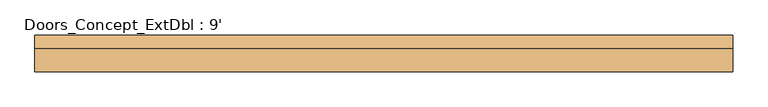
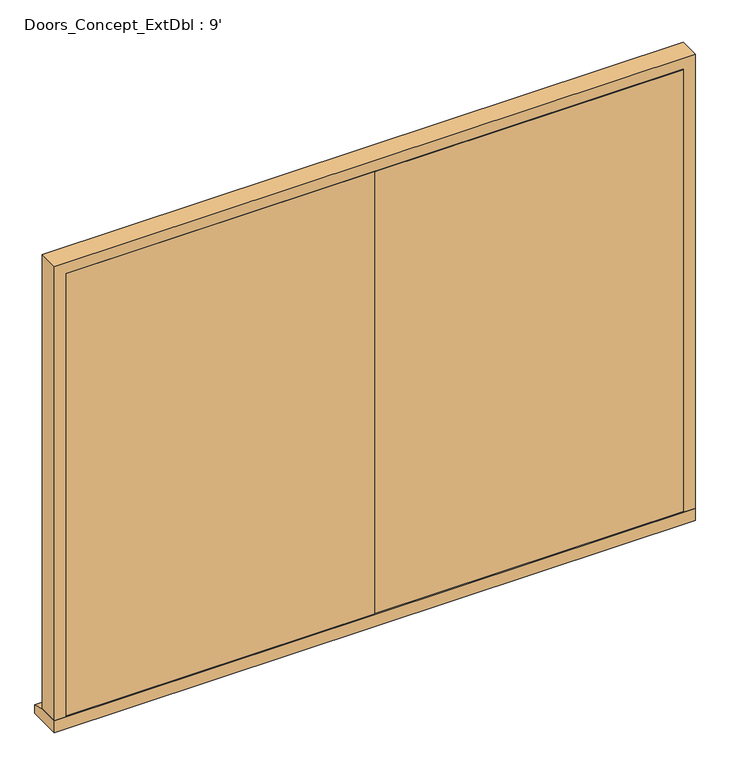
"""IFC4 building model written with IfcOpenShell, lengths in millimetres: door geometry, Doors_Concept_ExtDbl : 9'."""

from ifc_helpers import new_model, si_unit, frame, origin, place, context, project, spatial, polyline, outline, extrude, faceted_brep, source, transform, mapped, element, save


def doors_concept_extdbl_9_6115d45a(model_context):
    return source(origin(), model_context, "Body", "SolidModel", [
        faceted_brep([(1301.1, 74.06, 54.5), (1371.6, 74.06, 54.5), (1371.6, -14.94, 54.5), (1323.1, -14.94, 54.5), (1323.1, 32.06, 54.5), (1301.1, 32.06, 54.5), (1301.1, 74.06, 2039.5), (-1301.1, 74.06, 2039.5), (-1301.1, 74.06, 54.5), (-1371.6, 74.06, 54.5), (-1371.6, 74.06, 2110.0), (1371.6, 74.06, 2110.0), (1371.6, -14.94, 2110.0), (-1371.6, -14.94, 2110.0), (-1371.6, -14.94, 54.5), (-1323.1, -14.94, 54.5), (-1323.1, -14.94, 2061.5), (1323.1, -14.94, 2061.5), (1323.1, 32.06, 2061.5), (-1323.1, 32.06, 2061.5), (-1323.1, 32.06, 54.5), (-1301.1, 32.06, 54.5), (-1301.1, 32.06, 2039.5), (1301.1, 32.06, 2039.5)], [[[0, 1, 2, 3, 4, 5]], [[1, 0, 6, 7, 8, 9, 10, 11]], [[2, 1, 11, 12]], [[3, 2, 12, 13, 14, 15, 16, 17]], [[4, 3, 17, 18]], [[5, 4, 18, 19, 20, 21, 22, 23]], [[0, 5, 23, 6]], [[7, 22, 21, 8]], [[8, 21, 20, 15, 14, 9]], [[13, 10, 9, 14]], [[19, 16, 15, 20]], [[12, 11, 10, 13]], [[18, 17, 16, 19]], [[6, 23, 22, 7]]]),
        extrude(outline(polyline([(1320.1, -14.94), (1.5, -14.94), (1.5, 29.06), (1320.1, 29.06), (1320.1, -14.94)])), frame((0.0, 0.0, 58.5), z_axis=(0.0, 0.0, 1.0), x_axis=(1.0, 0.0, 0.0)), (0.0, 0.0, 1.0), 2000.0),
        extrude(outline(polyline([(-1.5, -14.94), (-1320.1, -14.94), (-1320.1, 29.06), (-1.5, 29.06), (-1.5, -14.94)])), frame((0.0, 0.0, 58.5), z_axis=(0.0, 0.0, 1.0), x_axis=(1.0, 0.0, 0.0)), (0.0, 0.0, 1.0), 2000.0),
        extrude(outline(polyline([(-14.94, 0.0), (-14.94, 54.5), (74.06, 54.5), (129.06, 38.5947221), (129.06, 0.0), (-14.94, 0.0)])), frame((-1371.6, 0.0, 0.0), z_axis=(1.0, 0.0, 0.0), x_axis=(0.0, 1.0, 0.0)), (0.0, 0.0, 1.0), 2743.2),
    ])


if __name__ == "__main__":
    model = new_model("IFC4")
    model_context = context("Model", 3, world=origin())
    ifc_project = project(units=[si_unit("LENGTHUNIT", "METRE", prefix="MILLI")], contexts=[model_context])
    site = spatial("IfcSite", under=ifc_project)
    building = spatial("IfcBuilding", under=site)
    placement = place(None, origin())
    doors_concept_extdbl_9_shape = doors_concept_extdbl_9_6115d45a(model_context)
    element("IfcDoor", 1, ObjectType="Doors_Concept_ExtDbl : 9'", at=placement, inside=building, context=model_context, shape_type="MappedRepresentation", body=[
        mapped(doors_concept_extdbl_9_shape, transform((0.0, 0.0, 0.0), x_axis=(1.0, 0.0, 0.0), y_axis=(0.0, 1.0, 0.0), z_axis=(0.0, 0.0, 1.0))),
    ])
    save(model, "model.ifc")

# Revit data of these elements
# Type "Doors_Concept_ExtDbl : 9'"
#   Type Mark = "54"
#   Type Comments = "External Double"
#   Operation = "DoubleDoorSingleSwing"
#   Construction Type Id = "GSP4R"
#   Keynote = "L10"
#   Analytic Construction = "1/8 in Pilkington single glazing"
#   Visual Light Transmittance = 0.9
#   Thickness = 0.144357 ft
#   Solar Heat Gain Coefficient = 0.78
#   Rough Width = 9.0 ft
#   Rough Height = 6.922572 ft
#   Heat Transfer Coefficient (U) = 3.6886 W/(m²·K)
#   FrameWidth = 0.137795 ft
#   FrameOffset - External = 0.082021 ft
#   Height = 6.922572 ft
#   Width = 9.0 ft
#   Define Thermal Properties by = 1
#   Function = 1
#   Material Door = Door - Glazing
#   Material Frame = Concept
#   Wall Closure = (empty or 0)
# Element 1 (IfcDoor, "Doors_Concept_ExtDbl : 9'")
#   Materials on its faces: "Concept", "Door - Glazing"
# Materials
#   "Door - Glazing": colour RGB 0 0 255, transparency 0.75
#   "Concept": colour RGB 128 128 255, transparency 0.5
